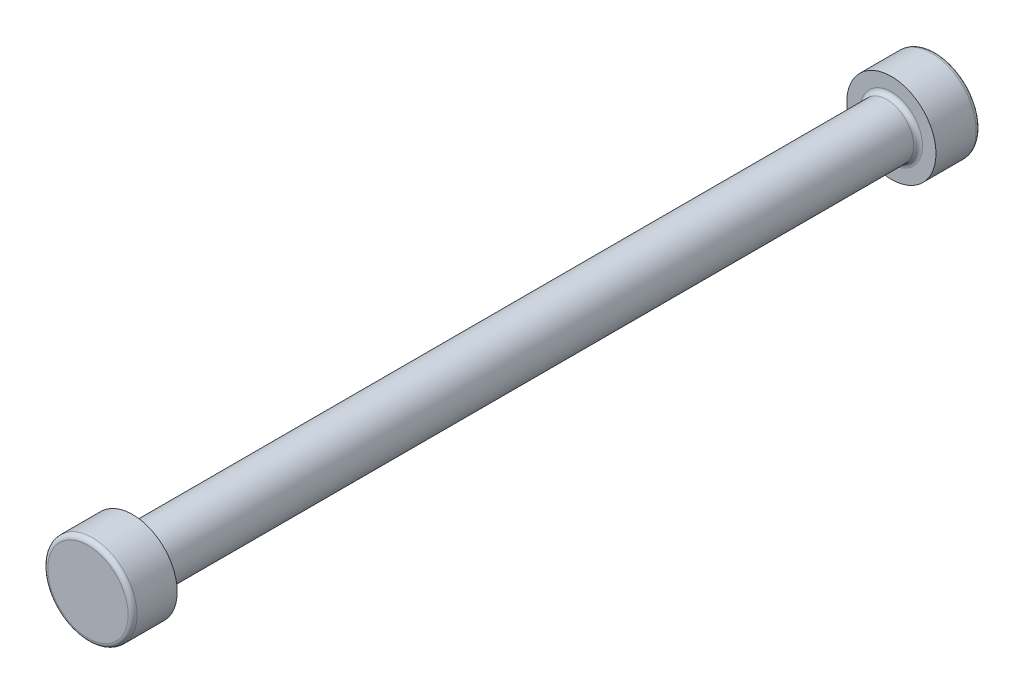
SolidWorks part; units mm, degrees
material "Plain Carbon Steel"
ref_plane "Front Plane" through (0, 0, 0) normal (0, 0, 1) x (1, 0, 0)
ref_plane "Top Plane" through (0, 0, 0) normal (0, 1, 0) x (1, 0, 0)
ref_plane "Right Plane" through (0, 0, 0) normal (1, 0, 0) x (0, 0, -1)
sketch "Shaft Profile Ø6" plane through (0, 0, 0) normal (0, 0, 1) x (1, 0, 0)
  circle A0 centre (0, 0) radius 3
  dimension "D1" = 6
extrude "Shaft Ø6x95" add sketch "Shaft Profile Ø6" along normal mid plane 95
sketch "Head Profile Ø10" plane through (0, 0, 47.5) normal (0, 0, 1) x (1, 0, 0)
  circle A0 centre (0, 0) radius 5
  dimension "D1" = 10
extrude "Head Ø10x5" add sketch "Head Profile Ø10" against normal blind 5
mirror "Head Mirror" about plane through (0, 0, 0) normal (0, 0, 1) of "Head Ø10x5"
fillet "Head Edge Fillets R0.5" radius 0.5 4 edges at (5, 0, -47.5) (5, 0, 47.5) (-3, 0, -42.5) (3, 0, 42.5)
